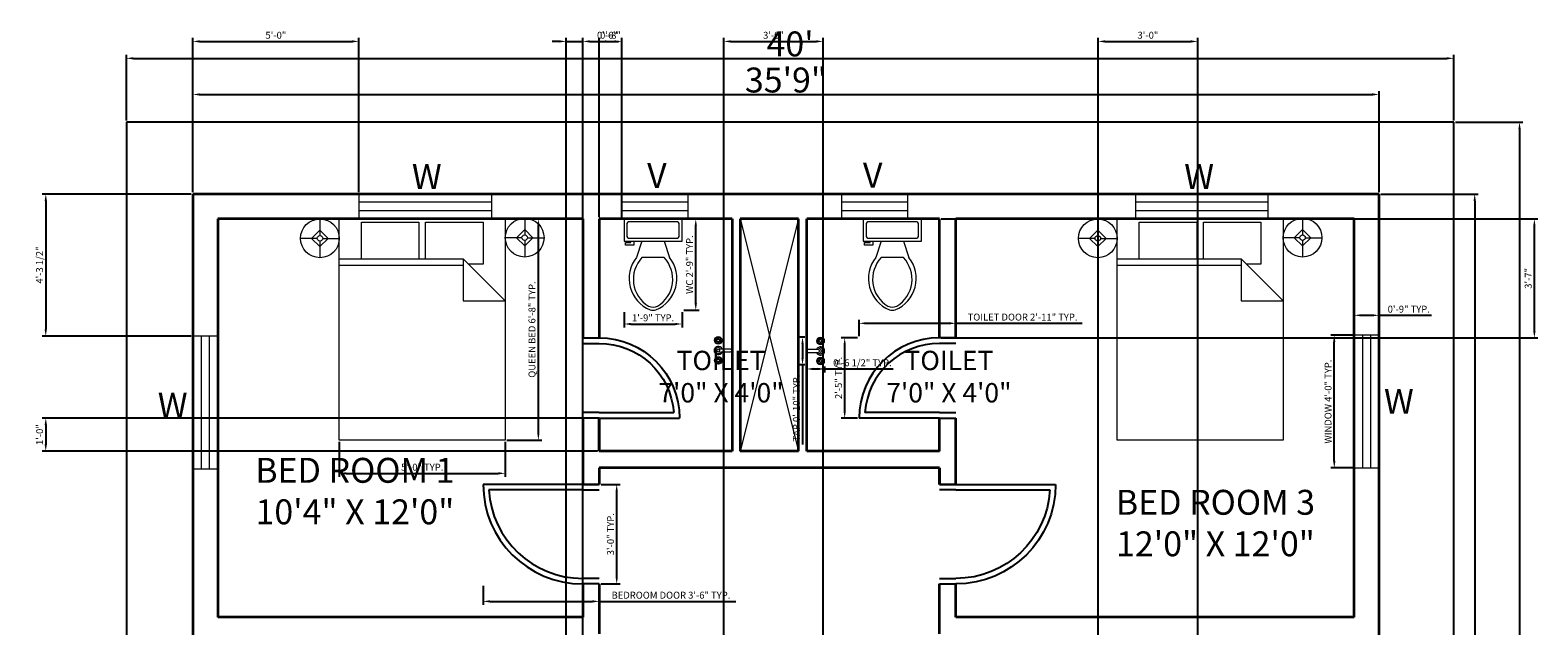
# Model space of a CAD drawing. Units: inches. Extents: x 1868 to 2413, y 1522 to 2138.
# Tile 4 of 4: x 1868 to 2413, y 1923 to 2138. Entities that reach past the tile are written whole.
import ezdxf

# ---------------------------------------------------------------- set-up
doc = ezdxf.new("R2010")
doc.units = ezdxf.units.IN
for name, color, linetype, lineweight in [('A-ANNO-DIMS', 2, 'Continuous', 18), ('A-ANNO-TEXT', 7, 'Continuous', 18), ('A-AREA-IDEN', 7, 'Continuous', 25), ('A-DOOR', 3, 'Continuous', 25), ('A-FLOR-FIXT', 9, 'Continuous', 18), ('A-FLOR-OPEN', 4, 'Continuous', 18), ('A-FURN', 8, 'Continuous', 18), ('A-GLAZ', 4, 'Continuous', 18), ('A-WALL', 7, 'Continuous', 35), ('C-PROP', 7, 'Continuous', 25)]:
    doc.layers.add(name, color=color, linetype=linetype, lineweight=lineweight)
doc.styles.get("Standard").update_dxf_attribs({"font": 'arial.ttf'})
doc.dimstyles.new('ISO-25', dxfattribs={"dimtxt": 2.5, "dimasz": 2.5, "dimexe": 1.25, "dimexo": 0.625, "dimtad": 1, "dimdec": 0, "dimlunit": 3, "dimtxsty": 'Standard', "dimcen": 2.5, "dimadec": 0, "dimazin": 0, "dimtfac": 1, "dimtdec": 0, "dimtmove": 0, "dimatfit": 3, "dimfxl": 1, "dimarcsym": 0})

# ---------------------------------------------------------------- blocks, each defined once
blk = doc.blocks.new('Lamp - Table')
for p, q in [((0, 7), (0, 1)), ((-1, 0), (-7, 0)), ((0, 3), (-3, 0)), ((-3, 0), (0, -3)), ((3, 0), (0, 3)), ((0, -3), (3, 0)), ((1, 0), (7, 0)), ((0, -1), (0, -7))]:
    blk.add_line(p, q)
for radius in [7, 1]:
    blk.add_circle((0, 0), radius)
blk = doc.blocks.new('Bed - Queen')
for p, q in [((0, -80.00003), (0, 0)), ((0, 0), (59.99999, 0)), ((59.99999, 0), (59.99999, -80.00003)), ((7.99999, -1.2), (28.79998, -1.2)), ((7.99999, -14.4), (7.99999, -1.2)), ((28.79998, -1.2), (28.79998, -14.4)), ((31.19999, -1.2), (51.99999, -1.2)), ((31.19999, -14.4), (31.19999, -1.2)), ((51.99999, -1.2), (51.99999, -16.4)), ((0, -14.4), (44.8, -14.4)), ((59.99999, -29.6), (44.8, -14.4)), ((44.8, -14.4), (44.8, -29.6)), ((44.8, -16.8), (0, -16.8)), ((51.99999, -16.4), (46.79936, -16.4)), ((44.8, -29.6), (59.99999, -29.6)), ((59.99999, -80.00003), (0, -80.00003))]:
    blk.add_line(p, q)
blk = doc.blocks.new('Toilet - top')
for p, q in [((9.5, -6), (9.5, -2)), ((-10, -8.5), (-8, -8.5)), ((-10, -9.5), (-10, -8.5)), ((-7, -9.5), (-10, -9.5)), ((-8, -8.5), (-8, -8)), ((-7, -8), (-7, -9.5)), ((-4, -8), (-6, -14)), ((4, -8), (6, -14)), ((4, -14), (-4, -14))]:
    blk.add_line(p, q)
blk.add_lwpolyline([(10.5, -8), (10.5, 0), (-10.5, 0), (-10.5, -8)], close=True)
for points in [[(-9.5, -2), (-9.5, -6)], [(8.5, -1), (-8.5, -1)], [(-8.5, -7), (8.5, -7)]]:
    blk.add_lwpolyline(points)
for centre, radius, start, end in [((-8.62, -1.88), 0.884, 81.8699, 188.1301), ((8.62, -1.88), 0.884, 351.8699, 98.1301), ((-8.62, -6.12), 0.884, 171.8699, 278.1301), ((8.62, -6.12), 0.884, 261.8699, 8.1301), ((3.52, -21.58), 12.17, 141.4691, 247.9714), ((4.2, -21.82), 11.33, 136.3677, 238.9468), ((-3.52, -21.58), 12.17, 292.0284, 38.5307), ((-4.2, -21.82), 11.33, 301.053, 43.6321), ((0, -27.88), 4, 245.7318, 294.2682), ((0, -29), 4, 254.8605, 285.1395)]:
    blk.add_arc(centre, radius, start, end)
blk = doc.blocks.new('Faucet - Bathroom top')
for p, q in [((-4.107, 0.125), (-4.375, 0.125)), ((-3.75, 0.4788), (-3.75, 0.75)), ((-3.5, 0.482), (-3.5, 0.75)), ((-3.1461, 0.125), (-2.875, 0.125)), ((3.143, 0.125), (2.875, 0.125)), ((3.5, 0.4788), (3.5, 0.75)), ((3.75, 0.482), (3.75, 0.75)), ((4.1039, 0.125), (4.375, 0.125)), ((-4.1039, -0.125), (-4.375, -0.125)), ((-3.75, -0.4821), (-3.75, -0.75)), ((-3.5, -0.4789), (-3.5, -0.75)), ((-3.143, -0.125), (-2.875, -0.125)), ((-0.5, -0.8639), (-0.5, -4.5)), ((0.5, -4.5), (0.5, -0.8631)), ((3.1461, -0.125), (2.875, -0.125)), ((3.5, -0.4821), (3.5, -0.75)), ((3.75, -0.4789), (3.75, -0.75)), ((4.107, -0.125), (4.375, -0.125))]:
    blk.add_line(p, q)
for centre, radius in [((-3.625, 0), 1.375), ((-4.625, 0), 0.2795), ((-3.625, 0), 0.5), ((-3.625, 1), 0.2795), ((-2.625, 0), 0.2795), ((0, 0), 0.5), ((3.625, 0), 1.375), ((2.625, 0), 0.2795), ((3.625, 0), 0.5), ((3.625, 1), 0.2795), ((4.625, 0), 0.2795), ((-3.625, -1), 0.2795), ((3.625, -1), 0.2795)]:
    blk.add_circle(centre, radius)
for centre, radius, start, end in [((-3.625, 0), 1, 105.2407, 164.2093), ((-3.625, 0), 1, 16.44125, 74.07887), ((0, 0), 1.5, 289.6514, 250.3603), ((0, 0), 1, 300.3431, 239.7554), ((3.625, 0), 1, 106.12, 164.0884), ((3.625, 0), 1, 16.23422, 73.90469), ((-3.625, 0), 1, 196.2342, 253.9047), ((-3.625, 0), 1, 286.12, 344.0884), ((0, -4.5), 0.5, 180, 0), ((3.625, 0), 1, 196.4413, 254.0789), ((3.625, 0), 1, 285.2407, 344.2093)]:
    blk.add_arc(centre, radius, start, end)
blk = doc.blocks.new('*D11')
at = {"layer": 'A-ANNO-DIMS', "color": 0, "lineweight": -2, "transparency": 16777216}
for p, q in [((1902.46, 2105.58), (1902.46, 2129.26)), ((1904.96, 2128.01), (2379.96, 2128.01)), ((2382.46, 2105.58), (2382.46, 2129.26))]:
    blk.add_line(p, q, dxfattribs=at)
at = {"layer": 'A-ANNO-DIMS', "color": 0, "transparency": 16777216}
for points in [[(1904.96, 2128.43), (1904.96, 2127.6), (1902.46, 2128.01)], [(2379.96, 2128.43), (2379.96, 2127.6), (2382.46, 2128.01)]]:
    blk.add_solid(points, dxfattribs=at)
at = {"layer": 'Defpoints', "color": 0, "transparency": 16777216}
for p in [(2382.46, 2128.01), (1902.46, 2104.95), (2382.46, 2104.95)]:
    blk.add_point(p, dxfattribs=at)
at = {"layer": 'A-ANNO-DIMS', "color": 0, "transparency": 16777216, "insert": (2142.46, 2133.23), "char_height": 2.5, "attachment_point": 5}
blk.add_mtext("{\\H3.6x;40'}", dxfattribs=at)
blk = doc.blocks.new('*D12')
at = {"layer": 'A-ANNO-DIMS', "color": 0, "lineweight": -2, "transparency": 16777216}
for p, q in [((2383.08, 2104.95), (2407.51, 2104.95)), ((2406.26, 2102.45), (2406.26, 1555.45)), ((2383.08, 1552.95), (2407.51, 1552.95))]:
    blk.add_line(p, q, dxfattribs=at)
at = {"layer": 'A-ANNO-DIMS', "color": 0, "transparency": 16777216}
for points in [[(2405.84, 2102.45), (2406.68, 2102.45), (2406.26, 2104.95)], [(2405.84, 1555.45), (2406.68, 1555.45), (2406.26, 1552.95)]]:
    blk.add_solid(points, dxfattribs=at)
at = {"layer": 'Defpoints', "color": 0, "transparency": 16777216}
for p in [(2382.46, 2104.95), (2382.46, 1552.95), (2406.26, 1552.95)]:
    blk.add_point(p, dxfattribs=at)
at = {"layer": 'A-ANNO-DIMS', "color": 0, "transparency": 16777216, "insert": (2401.04, 1828.95), "char_height": 2.5, "attachment_point": 5, "rotation": 90}
blk.add_mtext("{\\H3.6x;46'}", dxfattribs=at)
blk = doc.blocks.new('*D13')
at = {"layer": 'A-ANNO-DIMS', "color": 0, "lineweight": -2, "transparency": 16777216}
for p, q in [((1926.46, 2079.58), (1926.46, 2116.2)), ((2355.46, 2079.58), (2355.46, 2116.2)), ((1928.96, 2114.95), (2352.96, 2114.95))]:
    blk.add_line(p, q, dxfattribs=at)
at = {"layer": 'A-ANNO-DIMS', "color": 0, "transparency": 16777216}
for points in [[(1928.96, 2115.37), (1928.96, 2114.53), (1926.46, 2114.95)], [(2352.96, 2115.37), (2352.96, 2114.53), (2355.46, 2114.95)]]:
    blk.add_solid(points, dxfattribs=at)
at = {"layer": 'Defpoints', "color": 0, "transparency": 16777216}
for p in [(2355.46, 2114.95), (1926.46, 2078.95), (2355.46, 2078.95)]:
    blk.add_point(p, dxfattribs=at)
at = {"layer": 'A-ANNO-DIMS', "color": 0, "transparency": 16777216, "insert": (2140.96, 2120.17), "char_height": 2.5, "attachment_point": 5}
blk.add_mtext('{\\H3.6x;35\'9"}', dxfattribs=at)
blk = doc.blocks.new('*D14')
at = {"layer": 'A-ANNO-DIMS', "color": 0, "lineweight": -2, "transparency": 16777216}
for p, q in [((2356.08, 2078.95), (2391.3, 2078.95)), ((2390.05, 2076.45), (2390.05, 1591.45)), ((2356.08, 1588.95), (2391.3, 1588.95))]:
    blk.add_line(p, q, dxfattribs=at)
at = {"layer": 'A-ANNO-DIMS', "color": 0, "transparency": 16777216}
for points in [[(2389.63, 2076.45), (2390.46, 2076.45), (2390.05, 2078.95)], [(2389.63, 1591.45), (2390.46, 1591.45), (2390.05, 1588.95)]]:
    blk.add_solid(points, dxfattribs=at)
at = {"layer": 'Defpoints', "color": 0, "transparency": 16777216}
for p in [(2355.46, 2078.95), (2355.46, 1588.95), (2390.05, 1588.95)]:
    blk.add_point(p, dxfattribs=at)
at = {"layer": 'A-ANNO-DIMS', "color": 0, "transparency": 16777216, "insert": (2384.83, 1833.95), "char_height": 2.5, "attachment_point": 5, "rotation": 90}
blk.add_mtext('{\\H3.6x;40\'10"}', dxfattribs=at)
blk = doc.blocks.new('WIN-48IN')
for p, q in [((0, 48), (0, 0)), ((9, 48), (0, 48)), ((3, 48), (3, 0)), ((6, 0), (6, 48)), ((9, 0), (9, 48)), ((0, 0), (9, 0))]:
    blk.add_line(p, q)
blk = doc.blocks.new('VENT-24IN')
for p, q in [((24, 9), (0, 9)), ((0, 9), (0, 0)), ((24, 6), (0, 6)), ((24, 0), (24, 9)), ((0, 3), (24, 3)), ((0, 0), (24, 0))]:
    blk.add_line(p, q)
blk = doc.blocks.new('DOOR-36IN')
for p, q in [((36, 36), (0, 36)), ((0.06, 34), (0, 34)), ((36, 34), (2.06, 34)), ((36, 36), (42, 36)), ((36, 34), (42, 34)), ((42, 2), (36, 2)), ((42, 0), (36, 0))]:
    blk.add_line(p, q)
for radius, start in [(36, 180), (34, 183.3723)]:
    blk.add_arc((36, 36), radius, start, 270)
blk = doc.blocks.new('DOOR-29IN')
for p, q in [((35, 29), (29, 29)), ((35, 27), (29, 27)), ((0.07, 2), (0, 2)), ((29, 0), (0, 0)), ((29, 2), (2.07, 2)), ((29, 2), (35, 2)), ((29, 0), (35, 0))]:
    blk.add_line(p, q)
for radius, end in [(29, 180), (27, 175.752)]:
    blk.add_arc((29, 0), radius, 90, end)
blk = doc.blocks.new('*D24')
at = {"layer": 'A-ANNO-DIMS', "color": 0, "lineweight": -2, "transparency": 16777216}
for p, q in [((2345.83, 2027.89), (2338.01, 2027.89)), ((2339.26, 1982.39), (2339.26, 2025.39)), ((2345.83, 1979.89), (2338.01, 1979.89))]:
    blk.add_line(p, q, dxfattribs=at)
at = {"layer": 'A-ANNO-DIMS', "color": 0, "transparency": 16777216}
for points in [[(2338.84, 2025.39), (2339.67, 2025.39), (2339.26, 2027.89)], [(2338.84, 1982.39), (2339.67, 1982.39), (2339.26, 1979.89)]]:
    blk.add_solid(points, dxfattribs=at)
at = {"layer": 'Defpoints', "color": 0, "transparency": 16777216}
for p in [(2339.26, 2027.89), (2346.46, 2027.89), (2346.46, 1979.89)]:
    blk.add_point(p, dxfattribs=at)
at = {"layer": 'A-ANNO-DIMS', "color": 0, "transparency": 16777216, "insert": (2337.34, 2003.89), "char_height": 2.5, "attachment_point": 5, "rotation": 90}
blk.add_mtext('WINDOW 4\'-0" TYP.', dxfattribs=at)
blk = doc.blocks.new('*D25')
at = {"layer": 'A-ANNO-DIMS', "color": 0, "lineweight": -2, "transparency": 16777216}
for p, q in [((2346.46, 2028.51), (2346.46, 2036.34)), ((2348.96, 2035.09), (2352.96, 2035.09)), ((2355.46, 2028.51), (2355.46, 2036.34)), ((2355.46, 2035.09), (2374.45, 2035.09))]:
    blk.add_line(p, q, dxfattribs=at)
at = {"layer": 'A-ANNO-DIMS', "color": 0, "transparency": 16777216}
for points in [[(2348.96, 2035.5), (2348.96, 2034.67), (2346.46, 2035.09)], [(2352.96, 2035.5), (2352.96, 2034.67), (2355.46, 2035.09)]]:
    blk.add_solid(points, dxfattribs=at)
at = {"layer": 'Defpoints', "color": 0, "transparency": 16777216}
for p in [(2355.46, 2035.09), (2346.46, 2027.89), (2355.46, 2027.89)]:
    blk.add_point(p, dxfattribs=at)
at = {"layer": 'A-ANNO-DIMS', "color": 0, "transparency": 16777216, "insert": (2366.2, 2036.99), "char_height": 2.5, "attachment_point": 5}
blk.add_mtext('0\'-9" TYP.', dxfattribs=at)
blk = doc.blocks.new('*D28')
at = {"layer": 'A-ANNO-DIMS', "color": 0, "lineweight": -2, "transparency": 16777216}
for p, q in [((2031.46, 1937.33), (2031.46, 1930.4)), ((2073.46, 1937.33), (2073.46, 1930.4)), ((2033.96, 1931.65), (2070.96, 1931.65)), ((2073.46, 1931.65), (2122.8, 1931.65))]:
    blk.add_line(p, q, dxfattribs=at)
at = {"layer": 'A-ANNO-DIMS', "color": 0, "transparency": 16777216}
for points in [[(2033.96, 1932.07), (2033.96, 1931.23), (2031.46, 1931.65)], [(2070.96, 1932.07), (2070.96, 1931.23), (2073.46, 1931.65)]]:
    blk.add_solid(points, dxfattribs=at)
at = {"layer": 'Defpoints', "color": 0, "transparency": 16777216}
for p in [(2031.46, 1937.95), (2073.46, 1937.95), (2073.46, 1931.65)]:
    blk.add_point(p, dxfattribs=at)
at = {"layer": 'A-ANNO-DIMS', "color": 0, "transparency": 16777216, "insert": (2099.38, 1933.57), "char_height": 2.5, "attachment_point": 5}
blk.add_mtext('BEDROOM DOOR 3\'-6" TYP.', dxfattribs=at)
blk = doc.blocks.new('*D29')
at = {"layer": 'A-ANNO-DIMS', "color": 0, "lineweight": -2, "transparency": 16777216}
for p, q in [((2074.08, 1973.95), (2081.01, 1973.95)), ((2079.76, 1940.45), (2079.76, 1971.45)), ((2074.08, 1937.95), (2081.01, 1937.95))]:
    blk.add_line(p, q, dxfattribs=at)
at = {"layer": 'A-ANNO-DIMS', "color": 0, "transparency": 16777216}
for points in [[(2079.34, 1971.45), (2080.17, 1971.45), (2079.76, 1973.95)], [(2079.34, 1940.45), (2080.17, 1940.45), (2079.76, 1937.95)]]:
    blk.add_solid(points, dxfattribs=at)
at = {"layer": 'Defpoints', "color": 0, "transparency": 16777216}
for p in [(2073.46, 1973.95), (2079.76, 1973.95), (2073.46, 1937.95)]:
    blk.add_point(p, dxfattribs=at)
at = {"layer": 'A-ANNO-DIMS', "color": 0, "transparency": 16777216, "insert": (2077.85, 1955.95), "char_height": 2.5, "attachment_point": 5, "rotation": 90}
blk.add_mtext('3\'-0" TYP.', dxfattribs=at)
blk = doc.blocks.new('*D30')
at = {"layer": 'A-ANNO-DIMS', "color": 0, "lineweight": -2, "transparency": 16777216}
for p, q in [((2167.46, 2027.58), (2167.46, 2033.45)), ((2169.96, 2032.2), (2199.96, 2032.2)), ((2202.46, 2027.58), (2202.46, 2033.45)), ((2202.46, 2032.2), (2248.09, 2032.2))]:
    blk.add_line(p, q, dxfattribs=at)
at = {"layer": 'A-ANNO-DIMS', "color": 0, "transparency": 16777216}
for points in [[(2169.96, 2032.62), (2169.96, 2031.78), (2167.46, 2032.2)], [(2199.96, 2032.62), (2199.96, 2031.78), (2202.46, 2032.2)]]:
    blk.add_solid(points, dxfattribs=at)
at = {"layer": 'Defpoints', "color": 0, "transparency": 16777216}
for p in [(2202.46, 2032.2), (2167.46, 2026.95), (2202.46, 2026.95)]:
    blk.add_point(p, dxfattribs=at)
at = {"layer": 'A-ANNO-DIMS', "color": 0, "transparency": 16777216, "insert": (2226.53, 2034.12), "char_height": 2.5, "attachment_point": 5}
blk.add_mtext('TOILET DOOR 2\'-11" TYP.', dxfattribs=at)
blk = doc.blocks.new('*D31')
at = {"layer": 'A-ANNO-DIMS', "color": 0, "lineweight": -2, "transparency": 16777216}
for p, q in [((2166.83, 2026.95), (2160.96, 2026.95)), ((2162.21, 2000.45), (2162.21, 2024.45)), ((2166.83, 1997.95), (2160.96, 1997.95))]:
    blk.add_line(p, q, dxfattribs=at)
at = {"layer": 'A-ANNO-DIMS', "color": 0, "transparency": 16777216}
for points in [[(2161.79, 2024.45), (2162.62, 2024.45), (2162.21, 2026.95)], [(2161.79, 2000.45), (2162.62, 2000.45), (2162.21, 1997.95)]]:
    blk.add_solid(points, dxfattribs=at)
at = {"layer": 'Defpoints', "color": 0, "transparency": 16777216}
for p in [(2162.21, 2026.95), (2167.46, 2026.95), (2167.46, 1997.95)]:
    blk.add_point(p, dxfattribs=at)
at = {"layer": 'A-ANNO-DIMS', "color": 0, "transparency": 16777216, "insert": (2160.31, 2012.45), "char_height": 2.5, "attachment_point": 5, "rotation": 90}
blk.add_mtext('2\'-5" TYP.', dxfattribs=at)
blk = doc.blocks.new('*D34')
at = {"layer": 'A-ANNO-DIMS', "color": 0, "lineweight": -2, "transparency": 16777216}
for p, q in [((2040.06, 2069.95), (2052.68, 2069.95)), ((2051.43, 1992.45), (2051.43, 2067.45)), ((2040.06, 1989.95), (2052.68, 1989.95))]:
    blk.add_line(p, q, dxfattribs=at)
at = {"layer": 'A-ANNO-DIMS', "color": 0, "transparency": 16777216}
for points in [[(2051.02, 2067.45), (2051.85, 2067.45), (2051.43, 2069.95)], [(2051.02, 1992.45), (2051.85, 1992.45), (2051.43, 1989.95)]]:
    blk.add_solid(points, dxfattribs=at)
at = {"layer": 'Defpoints', "color": 0, "transparency": 16777216}
for p in [(2039.43, 2069.95), (2051.43, 2069.95), (2039.43, 1989.95)]:
    blk.add_point(p, dxfattribs=at)
at = {"layer": 'A-ANNO-DIMS', "color": 0, "transparency": 16777216, "insert": (2049.44, 2029.95), "char_height": 2.5, "attachment_point": 5, "rotation": 90}
blk.add_mtext('QUEEN BED 6\'-8" TYP.', dxfattribs=at)
blk = doc.blocks.new('*D35')
at = {"layer": 'A-ANNO-DIMS', "color": 0, "lineweight": -2, "transparency": 16777216}
for p, q in [((1979.43, 1989.33), (1979.43, 1976.7)), ((2039.43, 1989.33), (2039.43, 1976.7)), ((1981.93, 1977.95), (2036.93, 1977.95))]:
    blk.add_line(p, q, dxfattribs=at)
at = {"layer": 'A-ANNO-DIMS', "color": 0, "transparency": 16777216}
for points in [[(1981.93, 1978.37), (1981.93, 1977.53), (1979.43, 1977.95)], [(2036.93, 1978.37), (2036.93, 1977.53), (2039.43, 1977.95)]]:
    blk.add_solid(points, dxfattribs=at)
at = {"layer": 'Defpoints', "color": 0, "transparency": 16777216}
for p in [(1979.43, 1989.95), (2039.43, 1989.95), (2039.43, 1977.95)]:
    blk.add_point(p, dxfattribs=at)
at = {"layer": 'A-ANNO-DIMS', "color": 0, "transparency": 16777216, "insert": (2009.43, 1979.85), "char_height": 2.5, "attachment_point": 5}
blk.add_mtext('5\'-0" TYP.', dxfattribs=at)
blk = doc.blocks.new('*D38')
at = {"layer": 'A-ANNO-DIMS', "color": 0, "lineweight": -2, "transparency": 16777216}
for p, q in [((2104.03, 2069.95), (2109.61, 2069.95)), ((2108.36, 2039.4), (2108.36, 2067.45)), ((2104.03, 2036.9), (2109.61, 2036.9))]:
    blk.add_line(p, q, dxfattribs=at)
at = {"layer": 'A-ANNO-DIMS', "color": 0, "transparency": 16777216}
for points in [[(2107.94, 2067.45), (2108.77, 2067.45), (2108.36, 2069.95)], [(2107.94, 2039.4), (2108.77, 2039.4), (2108.36, 2036.9)]]:
    blk.add_solid(points, dxfattribs=at)
at = {"layer": 'Defpoints', "color": 0, "transparency": 16777216}
for p in [(2103.4, 2069.95), (2108.36, 2069.95), (2103.4, 2036.9)]:
    blk.add_point(p, dxfattribs=at)
at = {"layer": 'A-ANNO-DIMS', "color": 0, "transparency": 16777216, "insert": (2106.44, 2053.43), "char_height": 2.5, "attachment_point": 5, "rotation": 90}
blk.add_mtext('WC 2\'-9" TYP.', dxfattribs=at)
blk = doc.blocks.new('*D39')
at = {"layer": 'A-ANNO-DIMS', "color": 0, "lineweight": -2, "transparency": 16777216}
for p, q in [((2082.4, 2036.28), (2082.4, 2030.7)), ((2103.4, 2036.28), (2103.4, 2030.7)), ((2084.9, 2031.95), (2100.9, 2031.95))]:
    blk.add_line(p, q, dxfattribs=at)
at = {"layer": 'A-ANNO-DIMS', "color": 0, "transparency": 16777216}
for points in [[(2084.9, 2032.36), (2084.9, 2031.53), (2082.4, 2031.95)], [(2100.9, 2032.36), (2100.9, 2031.53), (2103.4, 2031.95)]]:
    blk.add_solid(points, dxfattribs=at)
at = {"layer": 'Defpoints', "color": 0, "transparency": 16777216}
for p in [(2082.4, 2036.9), (2103.4, 2036.9), (2103.4, 2031.95)]:
    blk.add_point(p, dxfattribs=at)
at = {"layer": 'A-ANNO-DIMS', "color": 0, "transparency": 16777216, "insert": (2092.9, 2033.85), "char_height": 2.5, "attachment_point": 5}
blk.add_mtext('1\'-9" TYP.', dxfattribs=at)
blk = doc.blocks.new('*D40')
at = {"layer": 'A-ANNO-DIMS', "color": 0, "lineweight": -2, "transparency": 16777216}
for p, q in [((2147.83, 2027.19), (2145.71, 2027.19)), ((2146.96, 2024.69), (2146.96, 2019.69)), ((2147.83, 2017.19), (2145.71, 2017.19)), ((2146.96, 2017.19), (2146.96, 1988.43))]:
    blk.add_line(p, q, dxfattribs=at)
at = {"layer": 'A-ANNO-DIMS', "color": 0, "transparency": 16777216}
for points in [[(2146.54, 2024.69), (2147.37, 2024.69), (2146.96, 2027.19)], [(2146.54, 2019.69), (2147.37, 2019.69), (2146.96, 2017.19)]]:
    blk.add_solid(points, dxfattribs=at)
at = {"layer": 'Defpoints', "color": 0, "transparency": 16777216}
for p in [(2148.46, 2027.19), (2146.96, 2017.19), (2148.46, 2017.19)]:
    blk.add_point(p, dxfattribs=at)
at = {"layer": 'A-ANNO-DIMS', "color": 0, "transparency": 16777216, "insert": (2145.06, 2001.56), "char_height": 2.5, "attachment_point": 5, "rotation": 90}
blk.add_mtext('TAP 0\'-10" TYP.', dxfattribs=at)
blk = doc.blocks.new('*D41')
at = {"layer": 'A-ANNO-DIMS', "color": 0, "lineweight": -2, "transparency": 16777216}
for p, q in [((2148.46, 2016.57), (2148.46, 2014.44)), ((2150.96, 2015.69), (2152.46, 2015.69)), ((2154.96, 2016.57), (2154.96, 2014.44)), ((2154.96, 2015.69), (2179.77, 2015.69))]:
    blk.add_line(p, q, dxfattribs=at)
at = {"layer": 'A-ANNO-DIMS', "color": 0, "transparency": 16777216}
for points in [[(2150.96, 2016.11), (2150.96, 2015.27), (2148.46, 2015.69)], [(2152.46, 2016.11), (2152.46, 2015.27), (2154.96, 2015.69)]]:
    blk.add_solid(points, dxfattribs=at)
at = {"layer": 'Defpoints', "color": 0, "transparency": 16777216}
for p in [(2148.46, 2017.19), (2154.96, 2017.19), (2154.96, 2015.69)]:
    blk.add_point(p, dxfattribs=at)
at = {"layer": 'A-ANNO-DIMS', "color": 0, "transparency": 16777216, "insert": (2168.61, 2017.61), "char_height": 2.5, "attachment_point": 5}
blk.add_mtext('0\'-6 1/2" TYP.', dxfattribs=at)
blk = doc.blocks.new('*D54')
at = {"layer": 'A-ANNO-DIMS', "color": 0, "lineweight": -2, "transparency": 16777216}
for p, q in [((2118.46, 1706.58), (2118.46, 2135.38)), ((2120.96, 2134.13), (2151.96, 2134.13)), ((2154.46, 1706.58), (2154.46, 2135.38))]:
    blk.add_line(p, q, dxfattribs=at)
at = {"layer": 'A-ANNO-DIMS', "color": 0, "transparency": 16777216}
for points in [[(2120.96, 2134.54), (2120.96, 2133.71), (2118.46, 2134.13)], [(2151.96, 2134.54), (2151.96, 2133.71), (2154.46, 2134.13)]]:
    blk.add_solid(points, dxfattribs=at)
at = {"layer": 'Defpoints', "color": 0, "transparency": 16777216}
for p in [(2154.46, 2134.13), (2118.46, 1705.95), (2154.46, 1705.95)]:
    blk.add_point(p, dxfattribs=at)
at = {"layer": 'A-ANNO-DIMS', "color": 0, "transparency": 16777216, "insert": (2136.46, 2136.03), "char_height": 2.5, "attachment_point": 5}
blk.add_mtext('3\'-0"', dxfattribs=at)
blk = doc.blocks.new('*D56')
at = {"layer": 'A-ANNO-DIMS', "color": 0, "lineweight": -2, "transparency": 16777216}
for p, q in [((2253.87, 1787.58), (2253.87, 2135.38)), ((2256.37, 2134.13), (2287.37, 2134.13)), ((2289.87, 1787.58), (2289.87, 2135.38))]:
    blk.add_line(p, q, dxfattribs=at)
at = {"layer": 'A-ANNO-DIMS', "color": 0, "transparency": 16777216}
for points in [[(2256.37, 2134.54), (2256.37, 2133.71), (2253.87, 2134.13)], [(2287.37, 2134.54), (2287.37, 2133.71), (2289.87, 2134.13)]]:
    blk.add_solid(points, dxfattribs=at)
at = {"layer": 'Defpoints', "color": 0, "transparency": 16777216}
for p in [(2289.87, 2134.13), (2253.87, 1786.95), (2289.87, 1786.95)]:
    blk.add_point(p, dxfattribs=at)
at = {"layer": 'A-ANNO-DIMS', "color": 0, "transparency": 16777216, "insert": (2271.87, 2136.03), "char_height": 2.5, "attachment_point": 5}
blk.add_mtext('3\'-0"', dxfattribs=at)
blk = doc.blocks.new('*D57')
at = {"layer": 'A-ANNO-DIMS', "color": 0, "lineweight": -2, "transparency": 16777216}
for p, q in [((1926.46, 2079.58), (1926.46, 2135.38)), ((1928.96, 2134.13), (1984.05, 2134.13)), ((1986.55, 2079.58), (1986.55, 2135.38))]:
    blk.add_line(p, q, dxfattribs=at)
at = {"layer": 'A-ANNO-DIMS', "color": 0, "transparency": 16777216}
for points in [[(1928.96, 2134.54), (1928.96, 2133.71), (1926.46, 2134.13)], [(1984.05, 2134.54), (1984.05, 2133.71), (1986.55, 2134.13)]]:
    blk.add_solid(points, dxfattribs=at)
at = {"layer": 'Defpoints', "color": 0, "transparency": 16777216}
for p in [(1986.55, 2134.13), (1926.46, 2078.95), (1986.55, 2078.95)]:
    blk.add_point(p, dxfattribs=at)
at = {"layer": 'A-ANNO-DIMS', "color": 0, "transparency": 16777216, "insert": (1956.5, 2136.03), "char_height": 2.5, "attachment_point": 5}
blk.add_mtext('5\'-0"', dxfattribs=at)
blk = doc.blocks.new('*D58')
at = {"layer": 'A-ANNO-DIMS', "color": 0, "lineweight": -2, "transparency": 16777216}
for p, q in [((1925.83, 2078.95), (1872.03, 2078.95)), ((1873.28, 2076.45), (1873.28, 2030.07)), ((1925.83, 2027.57), (1872.03, 2027.57))]:
    blk.add_line(p, q, dxfattribs=at)
at = {"layer": 'A-ANNO-DIMS', "color": 0, "transparency": 16777216}
for points in [[(1872.86, 2076.45), (1873.7, 2076.45), (1873.28, 2078.95)], [(1872.86, 2030.07), (1873.7, 2030.07), (1873.28, 2027.57)]]:
    blk.add_solid(points, dxfattribs=at)
at = {"layer": 'Defpoints', "color": 0, "transparency": 16777216}
for p in [(1926.46, 2078.95), (1873.28, 2027.57), (1926.46, 2027.57)]:
    blk.add_point(p, dxfattribs=at)
at = {"layer": 'A-ANNO-DIMS', "color": 0, "transparency": 16777216, "insert": (1871.36, 2053.26), "char_height": 2.5, "attachment_point": 5, "rotation": 90}
blk.add_mtext('4\'-3 1/2"', dxfattribs=at)
blk = doc.blocks.new('*D59')
at = {"layer": 'A-ANNO-DIMS', "color": 0, "lineweight": -2, "transparency": 16777216}
for p, q in [((2197.08, 2069.95), (2412.88, 2069.95)), ((2411.63, 2029.45), (2411.63, 2067.45)), ((2197.08, 2026.95), (2412.88, 2026.95))]:
    blk.add_line(p, q, dxfattribs=at)
at = {"layer": 'A-ANNO-DIMS', "color": 0, "transparency": 16777216}
for points in [[(2411.21, 2067.45), (2412.05, 2067.45), (2411.63, 2069.95)], [(2411.21, 2029.45), (2412.05, 2029.45), (2411.63, 2026.95)]]:
    blk.add_solid(points, dxfattribs=at)
at = {"layer": 'Defpoints', "color": 0, "transparency": 16777216}
for p in [(2196.46, 2069.95), (2411.63, 2069.95), (2196.46, 2026.95)]:
    blk.add_point(p, dxfattribs=at)
at = {"layer": 'A-ANNO-DIMS', "color": 0, "transparency": 16777216, "insert": (2409.73, 2048.45), "char_height": 2.5, "attachment_point": 5, "rotation": 90}
blk.add_mtext('3\'-7"', dxfattribs=at)
blk = doc.blocks.new('*D61')
at = {"layer": 'A-ANNO-DIMS', "color": 0, "lineweight": -2, "transparency": 16777216}
for p, q in [((2058.96, 2134.13), (2056.46, 2134.13)), ((2061.46, 1682.58), (2061.46, 2135.38)), ((2061.46, 2134.13), (2067.46, 2134.13)), ((2067.46, 1682.58), (2067.46, 2135.38)), ((2069.96, 2134.13), (2080.35, 2134.13))]:
    blk.add_line(p, q, dxfattribs=at)
at = {"layer": 'A-ANNO-DIMS', "color": 0, "transparency": 16777216}
for points in [[(2058.96, 2134.54), (2058.96, 2133.71), (2061.46, 2134.13)], [(2069.96, 2134.54), (2069.96, 2133.71), (2067.46, 2134.13)]]:
    blk.add_solid(points, dxfattribs=at)
at = {"layer": 'Defpoints', "color": 0, "transparency": 16777216}
for p in [(2067.46, 2134.13), (2061.46, 1681.95), (2067.46, 1681.95)]:
    blk.add_point(p, dxfattribs=at)
at = {"layer": 'A-ANNO-DIMS', "color": 0, "transparency": 16777216, "insert": (2076.4, 2136.03), "char_height": 2.5, "attachment_point": 5}
blk.add_mtext('0\'-6"', dxfattribs=at)
blk = doc.blocks.new('*D62')
at = {"layer": 'A-ANNO-DIMS', "color": 0, "lineweight": -2, "transparency": 16777216}
for p, q in [((2073.46, 2070.58), (2073.46, 2135.38)), ((2075.96, 2134.13), (2079.06, 2134.13)), ((2081.56, 2070.58), (2081.56, 2135.38))]:
    blk.add_line(p, q, dxfattribs=at)
at = {"layer": 'A-ANNO-DIMS', "color": 0, "transparency": 16777216}
for points in [[(2075.96, 2134.54), (2075.96, 2133.71), (2073.46, 2134.13)], [(2079.06, 2134.54), (2079.06, 2133.71), (2081.56, 2134.13)]]:
    blk.add_solid(points, dxfattribs=at)
at = {"layer": 'Defpoints', "color": 0, "transparency": 16777216}
for p in [(2081.56, 2134.13), (2073.46, 2069.95), (2081.56, 2069.95)]:
    blk.add_point(p, dxfattribs=at)
at = {"layer": 'A-ANNO-DIMS', "color": 0, "transparency": 16777216, "insert": (2077.51, 2136.03), "char_height": 2.5, "attachment_point": 5}
blk.add_mtext('0\'-8"', dxfattribs=at)
blk = doc.blocks.new('*D63')
at = {"layer": 'A-ANNO-DIMS', "color": 0, "lineweight": -2, "transparency": 16777216}
for p, q in [((2072.83, 1997.95), (1872.03, 1997.95)), ((1873.28, 1995.45), (1873.28, 1988.45)), ((2072.83, 1985.95), (1872.03, 1985.95))]:
    blk.add_line(p, q, dxfattribs=at)
at = {"layer": 'A-ANNO-DIMS', "color": 0, "transparency": 16777216}
for points in [[(1872.86, 1995.45), (1873.7, 1995.45), (1873.28, 1997.95)], [(1872.86, 1988.45), (1873.7, 1988.45), (1873.28, 1985.95)]]:
    blk.add_solid(points, dxfattribs=at)
at = {"layer": 'Defpoints', "color": 0, "transparency": 16777216}
for p in [(2073.46, 1997.95), (1873.28, 1985.95), (2073.46, 1985.95)]:
    blk.add_point(p, dxfattribs=at)
at = {"layer": 'A-ANNO-DIMS', "color": 0, "transparency": 16777216, "insert": (1871.38, 1991.95), "char_height": 2.5, "attachment_point": 5, "rotation": 90}
blk.add_mtext('1\'-0"', dxfattribs=at)

msp = doc.modelspace()

# ---------------------------------------------------------------- linework, layer by layer
at = {"layer": 'A-DOOR'}
for p, q in [((2073.46, 1973.95), (2067.46, 1973.95)), ((2067.46, 1973.95), (2067.46, 1973.95)), ((2196.46, 1973.95), (2202.46, 1973.95))]:
    msp.add_line(p, q, dxfattribs=at)
at = {"layer": 'A-FLOR-OPEN'}
for p, q in [((2145.46, 2069.95), (2124.46, 1985.95)), ((2124.46, 1985.95), (2124.46, 2069.95)), ((2124.46, 2069.95), (2145.46, 1985.95))]:
    msp.add_line(p, q, dxfattribs=at)
at = {"layer": 'A-WALL'}
for p, q in [((2355.46, 2078.95), (1926.46, 2078.95)), ((1926.46, 2078.95), (1926.46, 1588.95)), ((2355.46, 1588.95), (2355.46, 2078.95)), ((1935.46, 2069.95), (1935.46, 1925.95)), ((2067.46, 2069.95), (1935.46, 2069.95)), ((2067.46, 2069.95), (2067.46, 2026.95)), ((2073.46, 2069.95), (2073.46, 2026.95)), ((2121.46, 2069.95), (2073.46, 2069.95)), ((2121.46, 2069.95), (2121.46, 1985.95)), ((2124.46, 2069.95), (2124.46, 1985.95)), ((2145.46, 2069.95), (2124.46, 2069.95)), ((2145.46, 1985.95), (2145.46, 2069.95)), ((2148.46, 1985.95), (2148.46, 2069.95)), ((2196.46, 2069.95), (2148.46, 2069.95)), ((2196.46, 2026.95), (2196.46, 2069.95)), ((2346.46, 2069.95), (2202.46, 2069.95)), ((2202.46, 2026.95), (2202.46, 2069.95)), ((2346.46, 1925.95), (2346.46, 2069.95)), ((2067.46, 1997.95), (2067.46, 1973.95)), ((2073.46, 1985.95), (2073.46, 1997.95)), ((2073.46, 1997.95), (2073.46, 1985.95)), ((2196.46, 1985.95), (2196.46, 1997.95)), ((2196.46, 1985.95), (2196.46, 1997.95)), ((2202.46, 1973.95), (2202.46, 1997.95)), ((2121.46, 1985.95), (2073.46, 1985.95)), ((2145.46, 1985.95), (2124.46, 1985.95)), ((2196.46, 1985.95), (2148.46, 1985.95)), ((2196.46, 1979.95), (2073.46, 1979.95)), ((2073.46, 1979.95), (2073.46, 1973.95)), ((2073.46, 1979.95), (2073.46, 1973.95)), ((2196.46, 1979.95), (2196.46, 1973.95)), ((2196.46, 1973.95), (2196.46, 1979.95)), ((2067.46, 1937.95), (2067.46, 1925.95)), ((2073.46, 1937.95), (2073.46, 1919.95)), ((2196.46, 1919.95), (2196.46, 1937.95)), ((2202.46, 1925.95), (2202.46, 1937.95)), ((2067.46, 1925.95), (1935.46, 1925.95)), ((2346.46, 1925.95), (2202.46, 1925.95))]:
    msp.add_line(p, q, dxfattribs=at)
at = {"layer": 'C-PROP'}
for p, q in [((1902.46, 2104.95), (1902.46, 1552.95)), ((2382.46, 2104.95), (1902.46, 2104.95)), ((2382.46, 1552.95), (2382.46, 2104.95))]:
    msp.add_line(p, q, dxfattribs=at)

# ---------------------------------------------------------------- block references
at = {"layer": 'A-DOOR', "extrusion": (0, 0, -1), "zscale": -1}
for name, p in [('DOOR-29IN', (-2102.46, 1997.95)), ('DOOR-36IN', (-2238.46, 1937.95))]:
    msp.add_blockref(name, p, dxfattribs=at)
at = {"layer": 'A-DOOR'}
for name, p in [('DOOR-29IN', (2167.46, 1997.95)), ('DOOR-36IN', (2031.46, 1937.95))]:
    msp.add_blockref(name, p, dxfattribs=at)
at = {"layer": 'A-FLOR-FIXT'}
for p in [(2092.9, 2069.95), (2179.43, 2069.95)]:
    msp.add_blockref('Toilet - top', p, dxfattribs=at)
for p, rotation in [((2116.46, 2022.38), 90), ((2153.46, 2022.19), 270)]:
    msp.add_blockref('Faucet - Bathroom top', p, dxfattribs=dict(at, rotation=rotation))
at = {"layer": 'A-FURN'}
for name, p in [('Lamp - Table', (1972.44, 2062.92)), ('Bed - Queen', (1979.43, 2069.95)), ('Lamp - Table', (2046.48, 2063.16)), ('Lamp - Table', (2253.75, 2062.92)), ('Bed - Queen', (2260.74, 2069.95)), ('Lamp - Table', (2327.79, 2063.16))]:
    msp.add_blockref(name, p, dxfattribs=at)
at = {"layer": 'A-GLAZ'}
for p, rotation in [((1986.55, 2078.95), 270.0000000000002), ((2267.39, 2078.95), 270.0000000000004)]:
    msp.add_blockref('WIN-48IN', p, dxfattribs=dict(at, rotation=rotation))
for name, p in [('VENT-24IN', (2081.56, 2069.95)), ('VENT-24IN', (2161, 2069.95)), ('WIN-48IN', (1926.46, 1979.57)), ('WIN-48IN', (2346.46, 1979.89))]:
    msp.add_blockref(name, p, dxfattribs=at)

# ---------------------------------------------------------------- texts
at = {"layer": 'A-ANNO-TEXT', "char_height": 9, "attachment_point": 1}
for s, insert in [('\\pxqc;W', (1969.18, 2089.78)), ('\\pxqc;V', (2052.39, 2090.17)), ('\\pxqc;V', (2130.44, 2090.26)), ('\\pxqc;W', (2248.49, 2089.81)), ('\\pxqc;W', (1877.29, 2007.07)), ('\\pxqc;W', (2320.74, 2008.48))]:
    msp.add_mtext_dynamic_manual_height_columns(s, width=83.7859, gutter_width=12.5, heights=[0], dxfattribs=dict(at, insert=insert))
at = {"layer": 'A-AREA-IDEN', "char_height": 7, "attachment_point": 1}
for insert in [(2094.61, 2022.26), (2177.02, 2022.26)]:
    msp.add_mtext('\\pxqc;TOILET\\P7\'0" X 4\'0"', dxfattribs=dict(at, insert=insert))
at = {"layer": 'A-AREA-IDEN', "char_height": 9, "attachment_point": 1}
for s, insert in [('\\pxqc;BED ROOM 1\\P10\'4" X 12\'0"', (1938.86, 1983.54)), ('\\pxqc;BED ROOM 3\\P12\'0" X 12\'0"', (2250.07, 1971.98))]:
    msp.add_mtext_dynamic_manual_height_columns(s, width=92.4426, gutter_width=12.5, heights=[0], dxfattribs=dict(at, insert=insert))

# ---------------------------------------------------------------- dimensions: what is measured, and where the dimension line sits
at = {"layer": 'A-ANNO-DIMS'}
for base, p1, p2, text, override, picture, middle in [((2382.46, 2128.01), (1902.46, 2104.95), (2382.46, 2104.95), "{\\H3.6x;40'}", {"dimclrd": 0, "dimclre": 0, "dimclrt": 0}, '*D11', (2142.46, 2133.23)), ((2355.46, 2114.95), (1926.46, 2078.95), (2355.46, 2078.95), '{\\H3.6x;35\'9"}', {"dimclrd": 0, "dimclre": 0, "dimclrt": 0}, '*D13', (2140.96, 2120.17)), ((2202.46, 2032.2), (2167.46, 2026.95), (2202.46, 2026.95), 'TOILET DOOR <> TYP.', {"dimdec": 1, "dimlfac": 1, "dimrnd": 0, "dimzin": 1, "dimdsep": 46, "dimlunit": 4, "dimfrac": 2}, '*D30', (2226.53, 2034.12)), ((2355.46, 2035.09), (2346.46, 2027.89), (2355.46, 2027.89), '<> TYP.', {"dimdec": 1, "dimlfac": 1, "dimrnd": 0, "dimzin": 1, "dimdsep": 46, "dimlunit": 4, "dimfrac": 2}, '*D25', (2366.2, 2036.99)), ((2103.4, 2031.95), (2082.4, 2036.9), (2103.4, 2036.9), '<> TYP.', {"dimdec": 1, "dimlfac": 1, "dimrnd": 0, "dimzin": 1, "dimdsep": 46, "dimlunit": 4, "dimfrac": 2}, '*D39', (2092.9, 2033.85)), ((2154.96, 2015.69), (2148.46, 2017.19), (2154.96, 2017.19), '<> TYP.', {"dimdec": 1, "dimlfac": 1, "dimrnd": 0, "dimzin": 1, "dimdsep": 46, "dimlunit": 4, "dimfrac": 2}, '*D41', (2168.61, 2017.61)), ((2039.43, 1977.95), (1979.43, 1989.95), (2039.43, 1989.95), '<> TYP.', {"dimdec": 1, "dimlfac": 1, "dimrnd": 0, "dimzin": 1, "dimdsep": 46, "dimlunit": 4, "dimfrac": 2}, '*D35', (2009.43, 1979.85)), ((2073.46, 1931.65), (2031.46, 1937.95), (2073.46, 1937.95), 'BEDROOM DOOR <> TYP.', {"dimdec": 1, "dimlfac": 1, "dimrnd": 0, "dimzin": 1, "dimdsep": 46, "dimlunit": 4, "dimfrac": 2}, '*D28', (2099.38, 1933.57))]:
    dim = msp.add_linear_dim(base=base, p1=p1, p2=p2, text=text, dimstyle='ISO-25', override=override, dxfattribs=at)
    dim.commit()
    dim.dimension.update_dxf_attribs({"geometry": picture, "text_midpoint": middle})
for base, p1, p2, picture, middle in [((1986.55, 2134.13), (1926.46, 2078.95), (1986.55, 2078.95), '*D57', (1956.5, 2136.03)), ((2067.46, 2134.13), (2061.46, 1681.95), (2067.46, 1681.95), '*D61', (2076.4, 2136.03)), ((2081.56, 2134.13), (2073.46, 2069.95), (2081.56, 2069.95), '*D62', (2077.51, 2136.03)), ((2154.46, 2134.13), (2118.46, 1705.95), (2154.46, 1705.95), '*D54', (2136.46, 2136.03)), ((2289.87, 2134.13), (2253.87, 1786.95), (2289.87, 1786.95), '*D56', (2271.87, 2136.03))]:
    dim = msp.add_linear_dim(base=base, p1=p1, p2=p2, dimstyle='ISO-25', override={"dimdec": 1, "dimlfac": 1, "dimrnd": 0, "dimzin": 1, "dimdsep": 46, "dimlunit": 4, "dimfrac": 2}, dxfattribs=at)
    dim.commit()
    dim.dimension.update_dxf_attribs({"geometry": picture, "text_midpoint": middle})
for base, p1, p2, angle, text, override, picture, middle in [((2406.26, 1552.95), (2382.46, 2104.95), (2382.46, 1552.95), 90, "{\\H3.6x;46'}", {"dimclrd": 0, "dimclre": 0, "dimclrt": 0}, '*D12', (2401.04, 1828.95)), ((2390.05, 1588.95), (2355.46, 2078.95), (2355.46, 1588.95), 90, '{\\H3.6x;40\'10"}', {"dimclrd": 0, "dimclre": 0, "dimclrt": 0}, '*D14', (2384.83, 1833.95)), ((2051.43, 2069.95), (2039.43, 1989.95), (2039.43, 2069.95), 90, 'QUEEN BED <> TYP.', {"dimdec": 1, "dimlfac": 1, "dimrnd": 0, "dimzin": 1, "dimdsep": 46, "dimlunit": 4, "dimfrac": 2}, '*D34', (2049.44, 2029.95)), ((2108.3574, 2069.9511), (2103.4005, 2036.9048), (2103.4005, 2069.9511), 90, 'WC <> TYP.', {"dimdec": 1, "dimlfac": 1, "dimrnd": 0, "dimzin": 1, "dimdsep": 46, "dimlunit": 4, "dimfrac": 2}, '*D38', (2106.4398, 2053.428)), ((2146.96, 2017.19), (2148.46, 2027.19), (2148.46, 2017.19), 270, 'TAP <> TYP.', {"dimdec": 1, "dimlfac": 1, "dimrnd": 0, "dimzin": 1, "dimdsep": 46, "dimlunit": 4, "dimfrac": 2}, '*D40', (2145.06, 2001.56)), ((2162.21, 2026.95), (2167.46, 1997.95), (2167.46, 2026.95), 90, '<> TYP.', {"dimdec": 1, "dimlfac": 1, "dimrnd": 0, "dimzin": 1, "dimdsep": 46, "dimlunit": 4, "dimfrac": 2}, '*D31', (2160.31, 2012.45)), ((2339.26, 2027.89), (2346.46, 1979.89), (2346.46, 2027.89), 90, 'WINDOW <> TYP.', {"dimdec": 1, "dimlfac": 1, "dimrnd": 0, "dimzin": 1, "dimdsep": 46, "dimlunit": 4, "dimfrac": 2}, '*D24', (2337.34, 2003.89)), ((2079.76, 1973.95), (2073.46, 1937.95), (2073.46, 1973.95), 90, '<> TYP.', {"dimdec": 1, "dimlfac": 1, "dimrnd": 0, "dimzin": 1, "dimdsep": 46, "dimlunit": 4, "dimfrac": 2}, '*D29', (2077.85, 1955.95))]:
    dim = msp.add_linear_dim(base=base, p1=p1, p2=p2, angle=angle, text=text, dimstyle='ISO-25', override=override, dxfattribs=at)
    dim.commit()
    dim.dimension.update_dxf_attribs({"geometry": picture, "text_midpoint": middle})
for base, p1, p2, picture, middle in [((1873.28, 2027.57), (1926.46, 2078.95), (1926.46, 2027.57), '*D58', (1871.36, 2053.26)), ((2411.63, 2069.95), (2196.46, 2026.95), (2196.46, 2069.95), '*D59', (2409.73, 2048.45)), ((1873.28, 1985.95), (2073.46, 1997.95), (2073.46, 1985.95), '*D63', (1871.38, 1991.95))]:
    dim = msp.add_linear_dim(base=base, p1=p1, p2=p2, angle=90, dimstyle='ISO-25', override={"dimdec": 1, "dimlfac": 1, "dimrnd": 0, "dimzin": 1, "dimdsep": 46, "dimlunit": 4, "dimfrac": 2}, dxfattribs=at)
    dim.commit()
    dim.dimension.update_dxf_attribs({"geometry": picture, "text_midpoint": middle})

doc.saveas('drawing.dxf')
